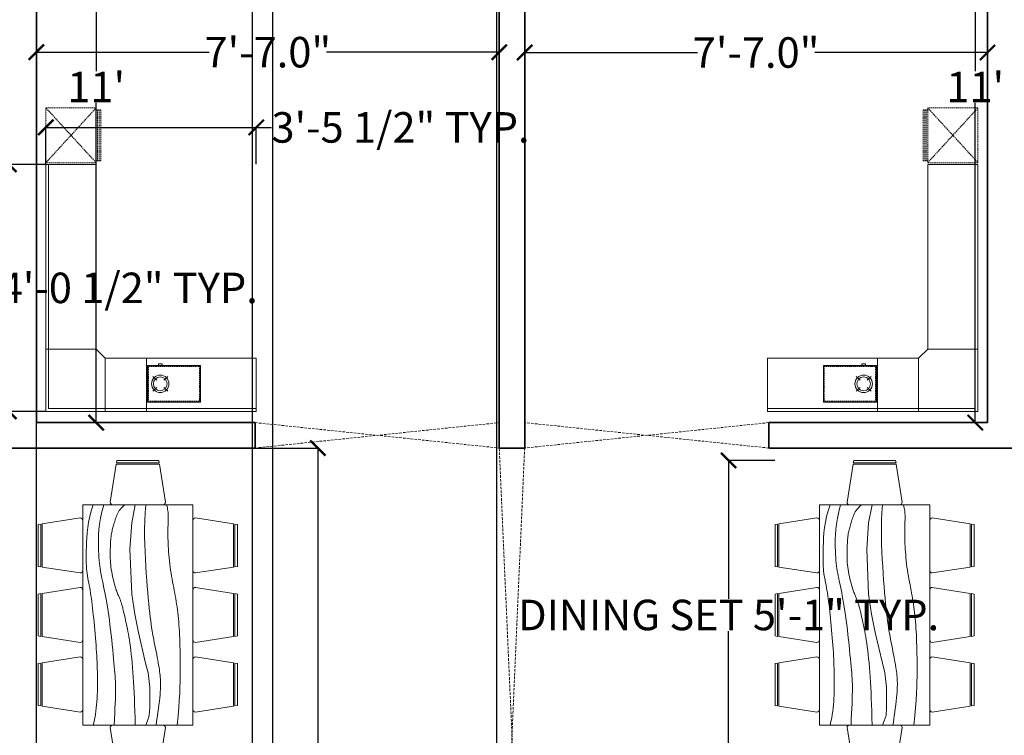
# Model space of a CAD drawing. Units: inches. Extents: x 844 to 2234, y 346 to 1084.
# Tile 44 of 93: x 1093 to 1287, y 823 to 964. Entities that reach past the tile are written whole.
import ezdxf

# ---------------------------------------------------------------- set-up
doc = ezdxf.new("R2010")
doc.units = ezdxf.units.IN
doc.header["$MEASUREMENT"] = 0
doc.linetypes.add('DASHED', pattern=[0.75, 0.5, -0.25])
doc.linetypes.add('HIDDEN', pattern=[0.375, 0.25, -0.125])
for name, color, linetype, lineweight in [('A-ANNO-DIMS', 2, 'Continuous', 18), ('A-EQPM', 42, 'Continuous', 18), ('A-EQPM-HIDN', 42, 'HIDDEN', 13), ('A-FLOR-CASE', 42, 'Continuous', 18), ('A-WALL', 7, 'Continuous', 35), ('A-WALL-OVHD', 7, 'DASHED', 18), ('furniture', 8, 'Continuous', 18)]:
    doc.layers.add(name, color=color, linetype=linetype, lineweight=lineweight)
doc.styles.add('ATTR', font='romans.shx', dxfattribs={"width": 0.8, "height": 0.7})
doc.styles.get("Standard").update_dxf_attribs({"font": 'arial.ttf'})
doc.dimstyles.get("Standard").update_dxf_attribs({"dimtxt": 6, "dimasz": 3, "dimexe": 0.18, "dimexo": 0.0625, "dimgap": 0.09, "dimtad": 0, "dimtih": 1, "dimtoh": 1, "dimdec": 1, "dimzin": 0, "dimdsep": 46, "dimlunit": 3, "dimtxsty": 'Standard', "dimblk": 'ARCHTICK', "dimcen": 0.09, "dimadec": 0, "dimazin": 0, "dimtfac": 1, "dimtdec": 1, "dimtofl": 0, "dimtmove": 0, "dimatfit": 3, "dimfxl": 1, "dimtolj": 1, "dimtzin": 0, "dimarcsym": 0})

# ---------------------------------------------------------------- blocks, each defined once
blk = doc.blocks.new('DIN42X84')
for p, q in [((-34.5377, 37.999999), (-34.6939, 37.000439)), ((-34.5377, 37.999999), (-18.5377, 37.999999)), ((-18.3814, 36.999659), (-18.5377, 37.999999)), ((-8.0001, 37.999999), (-8.1562, 37.000439)), ((-8.0001, 37.999999), (7.9999, 37.999999)), ((8.1562, 36.999659), (7.9999, 37.999999)), ((18.3813, 36.999659), (18.5376, 37.999999)), ((34.5376, 37.999999), (18.5376, 37.999999)), ((34.5376, 37.999999), (34.6938, 37.000439)), ((-34.772, 36.500609), (-37.0377, 21.999999)), ((-34.7681, 36.499999), (-18.2986, 36.499999)), ((-18.3793, 36.999999), (-34.6911, 36.999999)), ((-16.0377, 21.999999), (-18.3032, 36.499269)), ((-8.2343, 36.500609), (-10.5001, 21.999999)), ((-8.2305, 36.499999), (8.2391, 36.499999)), ((8.1584, 36.999999), (-8.1535, 36.999999)), ((10.4999, 21.999999), (8.2344, 36.499269)), ((16.0376, 21.999999), (18.3031, 36.499269)), ((34.768, 36.499999), (18.2985, 36.499999)), ((18.3792, 36.999999), (34.691, 36.999999)), ((34.7719, 36.500609), (37.0376, 21.999999)), ((-57.9997, 8.156299), (-59, 7.999989)), ((-59, -8.000011), (-59, 7.999989)), ((-58, 8.158429), (-58, -8.153391)), ((-57.5, -8.230411), (-57.5, 8.239139)), ((-43, 10.499989), (-57.4993, 8.234489)), ((43, 10.499989), (57.4992, 8.234489)), ((57.5, -8.230411), (57.5, 8.239139)), ((57.9996, 8.156299), (59, 7.999989)), ((58, 8.158429), (58, -8.153391)), ((59, -8.000011), (59, 7.999989)), ((-59, -8.000011), (-58.0005, -8.156181)), ((-57.5007, -8.234271), (-43, -10.500011)), ((57.5006, -8.234271), (43, -10.500011)), ((59, -8.000011), (58.0004, -8.156181)), ((-42, -21.000001), (42, -21.000001)), ((-34.772, -36.50061), (-37.0377, -22.000001)), ((-16.0377, -22.000001), (-18.3032, -36.499267)), ((-8.2343, -36.50061), (-10.5001, -22.000001)), ((10.4999, -22.000001), (8.2344, -36.499267)), ((16.0376, -22.000001), (18.3031, -36.499267)), ((34.7719, -36.50061), (37.0376, -22.000001)), ((-34.7681, -36.499999), (-18.2986, -36.499999)), ((-34.5377, -37.999999), (-34.6939, -37.000442)), ((-18.3793, -36.999999), (-34.6911, -36.999999)), ((-18.3814, -36.999664), (-18.5377, -37.999999)), ((-8.2305, -36.499999), (8.2391, -36.499999)), ((-8.0001, -37.999999), (-8.1562, -37.000442)), ((8.1584, -36.999999), (-8.1535, -36.999999)), ((8.1562, -36.999664), (7.9999, -37.999999)), ((34.768, -36.499999), (18.2985, -36.499999)), ((18.3792, -36.999999), (34.691, -36.999999)), ((18.3813, -36.999664), (18.5376, -37.999999)), ((34.5376, -37.999999), (34.6938, -37.000442)), ((-34.5377, -37.999999), (-18.5377, -37.999999)), ((-8.0001, -37.999999), (7.9999, -37.999999)), ((34.5376, -37.999999), (18.5376, -37.999999))]:
    blk.add_line(p, q)
for points in [[(-42, -21.000001), (-42, 20.999989), (42, 20.999989), (42, -21.000001)], [(-42, 16.999989), (-40.5974, 16.672209), (-39.2569, 16.395939), (-37.9668, 16.166109), (-36.7153, 15.977689), (-35.4906, 15.825599), (-34.281, 15.704799), (-33.0745, 15.610229), (-31.8595, 15.536839), (-30.6267, 15.480229), (-29.3778, 15.438619), (-28.117, 15.410889), (-26.8486, 15.395929), (-25.5767, 15.392599), (-24.3058, 15.399809), (-23.0399, 15.416409), (-21.7833, 15.441309), (-20.5384, 15.473619), (-19.2994, 15.513549), (-18.0587, 15.561549), (-16.8087, 15.618049), (-15.5417, 15.683499), (-14.25, 15.758369), (-12.9261, 15.843079), (-11.5622, 15.938089), (-10.1541, 16.043559), (-8.7108, 16.158419), (-7.2445, 16.281349), (-5.7675, 16.410999), (-4.2923, 16.546019), (-2.8311, 16.685069), (-1.3963, 16.826809), (0, 16.969889), (1.3474, 17.113339), (2.6447, 17.257689), (3.8928, 17.403829), (5.0924, 17.552659), (6.2444, 17.705069), (7.3498, 17.861959), (8.4092, 18.024219), (9.4237, 18.192759), (10.3952, 18.367629), (11.3311, 18.545639), (12.2397, 18.722759), (13.1297, 18.894949), (14.0095, 19.058179), (14.8876, 19.208429), (15.7725, 19.341659), (16.6727, 19.453839), (17.5977, 19.541909), (18.5617, 19.606689), (19.5795, 19.649979), (20.6664, 19.673569), (21.8374, 19.679239), (23.1076, 19.668789), (24.492, 19.644009), (26.0058, 19.606689), (27.6589, 19.554579), (29.4413, 19.469229), (31.3377, 19.328169), (33.3331, 19.108889), (35.4121, 18.788919), (37.5598, 18.345779), (39.7608, 17.756959), (42, 16.999989)], [(42, 12.999999), (39.3635, 13.704689), (36.9303, 14.232849), (34.6868, 14.608169), (32.6195, 14.854319), (30.7149, 14.994989), (28.9596, 15.053859), (27.34, 15.054629), (25.8427, 15.020959), (24.4543, 14.972439), (23.1628, 14.912279), (21.9562, 14.839589), (20.8227, 14.753449), (19.7504, 14.652989), (18.7273, 14.537299), (17.7416, 14.405489), (16.7814, 14.256669), (15.8348, 14.090369), (14.8899, 13.907959), (13.9348, 13.711209), (12.9575, 13.501929), (11.9464, 13.281899), (10.8893, 13.052909), (9.7745, 12.816759), (8.59, 12.575229), (7.3261, 12.330049), (5.9815, 12.082619), (4.557, 11.834299), (3.0536, 11.586429), (1.472, 11.340349), (-0.187, 11.097409), (-1.9223, 10.858939), (-3.7333, 10.626289), (-5.6141, 10.400739), (-7.539, 10.183249), (-9.4776, 9.974709), (-11.3991, 9.776019), (-13.2731, 9.588079), (-15.0689, 9.411789), (-16.756, 9.248039), (-18.3038, 9.097709), (-19.6928, 8.961719), (-20.9483, 8.840959), (-22.1065, 8.736319), (-23.2037, 8.648689), (-24.2763, 8.578979), (-25.3606, 8.528079), (-26.4928, 8.496879), (-27.7094, 8.486279), (-29.0411, 8.496689), (-30.4965, 8.526549), (-32.0787, 8.573829), (-33.7908, 8.636479), (-35.6359, 8.712459), (-37.6171, 8.799739), (-39.7374, 8.896259), (-42, 8.999999)], [(-42, 0.999999), (-39.2567, 1.059739), (-36.6668, 1.127399), (-34.2177, 1.203389), (-31.897, 1.288099), (-29.6923, 1.381949), (-27.5912, 1.485329), (-25.5812, 1.598659), (-23.65, 1.722319), (-21.7874, 1.856519), (-19.9935, 2.000569), (-18.2704, 2.153579), (-16.6207, 2.314649), (-15.0465, 2.482879), (-13.5503, 2.657379), (-12.1344, 2.837259), (-10.8011, 3.021619), (-9.5514, 3.209479), (-8.3812, 3.399579), (-7.2848, 3.590579), (-6.2569, 3.781129), (-5.2918, 3.969889), (-4.384, 4.155509), (-3.5281, 4.336659), (-2.7184, 4.511979), (-1.9505, 4.680359), (-1.2233, 4.841579), (-0.5369, 4.995629), (0.1087, 5.142519), (0.7135, 5.282239), (1.2776, 5.414799), (1.8009, 5.540189), (2.2834, 5.658409), (2.7259, 5.769699), (3.1323, 5.875159), (3.5073, 5.976139), (3.8555, 6.073989), (4.1816, 6.170049), (4.4904, 6.265659), (4.7863, 6.362169), (5.0742, 6.460919), (5.3584, 6.563099), (5.6417, 6.669299), (5.9267, 6.779989), (6.216, 6.895609), (6.512, 7.016589), (6.8174, 7.143399), (7.1347, 7.276479), (7.4664, 7.416279), (7.8159, 7.563169), (8.1896, 7.717219), (8.5948, 7.878439), (9.0386, 8.046819), (9.5282, 8.222369), (10.071, 8.405079), (10.674, 8.594959), (11.3446, 8.791999), (12.0866, 8.995459), (12.8902, 9.201609), (13.7421, 9.405969), (14.6294, 9.604059), (15.5387, 9.791399), (16.4569, 9.963509), (17.3709, 10.115919), (18.2674, 10.244149), (19.1361, 10.344989), (19.9772, 10.420299), (20.7936, 10.473209), (21.5884, 10.506879), (22.3645, 10.524419), (23.1248, 10.528969), (23.8725, 10.523669), (24.6103, 10.511649), (25.3403, 10.495379), (26.0601, 10.474629), (26.7663, 10.448509), (27.4556, 10.416119), (28.1244, 10.376559), (28.7695, 10.328939), (29.3873, 10.272359), (29.9746, 10.205939), (30.5293, 10.129059), (31.0552, 10.042329), (31.5572, 9.946639), (32.0406, 9.842899), (32.5104, 9.731989), (32.9716, 9.614799), (33.4295, 9.492249), (33.8891, 9.365219), (34.3546, 9.234229), (34.8266, 9.098309), (35.3051, 8.956129), (35.7897, 8.806329), (36.2802, 8.647569), (36.7765, 8.478519), (37.2783, 8.297819), (37.7854, 8.104139), (38.2976, 7.894309), (38.8146, 7.657969), (39.3361, 7.382899), (39.8617, 7.056919), (40.3912, 6.667829), (40.9243, 6.203449), (41.4607, 5.651569), (42, 4.999999)], [(42, 0.999999), (35.1214, 2.295539), (25.1178, 2.983399), (7.9376, 2.295539), (0.3261, 1.149099), (-6.6329, -0.226611), (-18.3763, -2.978061), (-22.0733, -3.895201), (-27.5101, -4.583071), (-32.9468, -4.583071), (-35.339, -4.583071), (-38.3836, -4.353771), (-40.3408, -3.665921), (-42, -3.000001)], [(42, -3.000001), (38.9344, -2.781351), (35.8829, -2.650251), (32.8567, -2.595491), (29.8672, -2.605821), (26.9257, -2.670031), (24.0436, -2.776881), (21.2323, -2.915141), (18.5031, -3.073591), (15.8668, -3.242611), (13.3327, -3.419021), (10.9095, -3.601241), (8.6059, -3.787731), (6.4305, -3.976901), (4.3921, -4.167191), (2.4994, -4.357031), (0.7611, -4.544851), (-0.8196, -4.729651), (-2.2614, -4.912671), (-3.5885, -5.095681), (-4.8252, -5.280481), (-5.9956, -5.468861), (-7.1239, -5.662621), (-8.2344, -5.863551), (-9.3513, -6.073431), (-10.4925, -6.293091), (-11.6511, -6.519461), (-12.814, -6.748531), (-13.968, -6.976251), (-15.0999, -7.198591), (-16.1965, -7.411531), (-17.2447, -7.611041), (-18.2313, -7.793081), (-19.1472, -7.954521), (-19.9994, -8.095811), (-20.7989, -8.218291), (-21.5568, -8.323311), (-22.2841, -8.412201), (-22.9919, -8.486311), (-23.6912, -8.546991), (-24.393, -8.595581), (-25.1087, -8.632751), (-25.8513, -8.656491), (-26.6337, -8.664101), (-27.4693, -8.652901), (-28.3711, -8.620211), (-29.3523, -8.563341), (-30.4262, -8.479601), (-31.6057, -8.366301), (-32.8956, -8.222561), (-34.2657, -8.054761), (-35.6772, -7.871051), (-37.0913, -7.679611), (-38.4695, -7.488621), (-39.7728, -7.306241), (-40.9626, -7.140641), (-42, -7.000001)], [(-42, -15.000001), (-38.4722, -15.350691), (-35.3039, -15.623741), (-32.4544, -15.828971), (-29.8831, -15.976191), (-27.5493, -16.075201), (-25.4123, -16.135831), (-23.4313, -16.167881), (-21.5659, -16.181151), (-19.7812, -16.183881), (-18.0665, -16.177871), (-16.4173, -16.163351), (-14.8288, -16.140551), (-13.2964, -16.109691), (-11.8154, -16.070991), (-10.3811, -16.024671), (-8.9888, -15.970971), (-7.6345, -15.909991), (-6.3163, -15.841401), (-5.0329, -15.764751), (-3.7831, -15.679591), (-2.5656, -15.585471), (-1.3791, -15.481951), (-0.2223, -15.368571), (0.9061, -15.244901), (2.0079, -15.110631), (3.0876, -14.966051), (4.1503, -14.811631), (5.2011, -14.647801), (6.2451, -14.475011), (7.2875, -14.293721), (8.3332, -14.104361), (9.3874, -13.907391), (10.4544, -13.703711), (11.5349, -13.495991), (12.6291, -13.287381), (13.7368, -13.081011), (14.8581, -12.880011), (15.9931, -12.687521), (17.1416, -12.506671), (18.3037, -12.340601), (19.4778, -12.191771), (20.6562, -12.059961), (21.8295, -11.944271), (22.9884, -11.843811), (24.1234, -11.757681), (25.2254, -11.684981), (26.2848, -11.624831), (27.2925, -11.576311), (28.2412, -11.538551), (29.1325, -11.510631), (29.9703, -11.491671), (30.7584, -11.480781), (31.5007, -11.477041), (32.2009, -11.479581), (32.8628, -11.487491), (33.4904, -11.499881), (34.0874, -11.515741), (34.6576, -11.533621), (35.2049, -11.551941), (35.733, -11.569151), (36.2459, -11.583661), (36.7473, -11.593931), (37.2411, -11.598371), (37.7311, -11.595421), (38.2211, -11.583281), (38.7152, -11.559251), (39.2177, -11.520361), (39.7326, -11.463671), (40.2641, -11.386241), (40.8164, -11.285111), (41.3937, -11.157351), (42, -11.000001)]]:
    blk.add_lwpolyline(points)
for centre, start, end in [((-36.0377, 21.999999), 180, 270), ((-17.0377, 21.999999), 270, 0), ((-9.5001, 21.999999), 180, 270), ((9.4999, 21.999999), 270, 0), ((17.0376, 21.999999), 180, 270), ((36.0376, 21.999999), 270, 0), ((-43, 9.499989), 0.00000068, 90), ((43, 9.499989), 90, 180), ((-43, -9.500011), 270, 0.00000068), ((43, -9.500011), 180, 270), ((-36.0377, -22.000001), 90, 180), ((-17.0377, -22.000001), 0, 90), ((-9.5001, -22.000001), 90, 180), ((9.4999, -22.000001), 0, 90), ((17.0376, -22.000001), 90, 180), ((36.0376, -22.000001), 0, 90)]:
    blk.add_arc(centre, 1, start, end)
at = {"style": 'ATTR', "width": 0.8, "flags": 9}
blk.add_attdef('ESTCODE', (0, 0), '', height=0.7, dxfattribs=at)
blk = doc.blocks.new('_ArchTick')
at = {"color": 0, "linetype": 'ByBlock', "const_width": 0.15}
blk.add_lwpolyline([(-0.5, -0.5), (0.5, 0.5)], dxfattribs=at)
blk = doc.blocks.new('*D25')
at = {"layer": 'A-ANNO-DIMS', "color": 0, "lineweight": -2, "transparency": 16777216}
for p, q in [((1096.62, 957.17), (1130.58, 957.17)), ((1096.62, 957.1), (1096.62, 956.99)), ((1187.62, 957.17), (1153.65, 957.17)), ((1187.62, 957.23), (1187.62, 957.35))]:
    blk.add_line(p, q, dxfattribs=at)
at = {"layer": 'Defpoints', "color": 0, "transparency": 16777216}
for p in [(1096.62, 957.17), (1187.62, 957.17), (1187.62, 957.17)]:
    blk.add_point(p, dxfattribs=at)
at = {"layer": 'A-ANNO-DIMS', "color": 0, "lineweight": -2, "transparency": 16777216, "xscale": 3, "yscale": 3, "zscale": 3, "rotation": 180}
blk.add_blockref('_ArchTick', (1096.62, 957.17), dxfattribs=at)
at = {"layer": 'A-ANNO-DIMS', "color": 0, "lineweight": -2, "transparency": 16777216, "xscale": 3, "yscale": 3, "zscale": 3}
blk.add_blockref('_ArchTick', (1187.62, 957.17), dxfattribs=at)
at = {"layer": 'A-ANNO-DIMS', "color": 0, "transparency": 16777216, "insert": (1142.12, 957.17), "char_height": 6, "attachment_point": 5}
blk.add_mtext('\\A1;7\'-7.0"', dxfattribs=at)
blk = doc.blocks.new('*D26')
at = {"layer": 'A-ANNO-DIMS', "color": 0, "lineweight": -2, "transparency": 16777216}
for p, q in [((1099.7, 1016.31), (1108.56, 1016.31)), ((1108.38, 1016.31), (1108.38, 953.41)), ((1108.38, 884.31), (1108.38, 947.21)), ((1099.7, 884.31), (1108.56, 884.31))]:
    blk.add_line(p, q, dxfattribs=at)
at = {"layer": 'Defpoints', "color": 0, "transparency": 16777216}
for p in [(1099.64, 1016.31), (1099.64, 884.31), (1108.38, 884.31)]:
    blk.add_point(p, dxfattribs=at)
at = {"layer": 'A-ANNO-DIMS', "color": 0, "lineweight": -2, "transparency": 16777216, "xscale": 3, "yscale": 3, "zscale": 3}
for p, rotation in [((1108.38, 1016.31), 90), ((1108.38, 884.31), 270)]:
    blk.add_blockref('_ArchTick', p, dxfattribs=dict(at, rotation=rotation))
at = {"layer": 'A-ANNO-DIMS', "color": 0, "transparency": 16777216, "insert": (1108.38, 950.31), "char_height": 6, "attachment_point": 5}
blk.add_mtext("\\A1;11'", dxfattribs=at)
blk = doc.blocks.new('*D27')
at = {"layer": 'A-ANNO-DIMS', "color": 0, "lineweight": -2, "transparency": 16777216}
for p, q in [((1283.21, 1016.31), (1281.03, 1016.31)), ((1281.21, 1016.31), (1281.21, 953.41)), ((1281.21, 884.31), (1281.21, 947.21)), ((1283.21, 884.31), (1281.03, 884.31))]:
    blk.add_line(p, q, dxfattribs=at)
at = {"layer": 'Defpoints', "color": 0, "transparency": 16777216}
for p in [(1283.27, 1016.31), (1281.21, 884.31), (1283.27, 884.31)]:
    blk.add_point(p, dxfattribs=at)
at = {"layer": 'A-ANNO-DIMS', "color": 0, "lineweight": -2, "transparency": 16777216, "xscale": 3, "yscale": 3, "zscale": 3}
for p, rotation in [((1281.21, 1016.31), 90), ((1281.21, 884.31), 270)]:
    blk.add_blockref('_ArchTick', p, dxfattribs=dict(at, rotation=rotation))
at = {"layer": 'A-ANNO-DIMS', "color": 0, "transparency": 16777216, "insert": (1281.21, 950.31), "char_height": 6, "attachment_point": 5}
blk.add_mtext("\\A1;11'", dxfattribs=at)
blk = doc.blocks.new('*D28')
at = {"layer": 'A-ANNO-DIMS', "color": 0, "lineweight": -2, "transparency": 16777216}
for p, q in [((1192.62, 957.17), (1192.62, 957.28)), ((1192.62, 957.1), (1226.58, 957.1)), ((1283.62, 957.1), (1249.65, 957.1)), ((1283.62, 957.17), (1283.62, 957.28))]:
    blk.add_line(p, q, dxfattribs=at)
at = {"layer": 'Defpoints', "color": 0, "transparency": 16777216}
for p in [(1192.62, 957.1), (1283.62, 957.1), (1283.62, 957.1)]:
    blk.add_point(p, dxfattribs=at)
at = {"layer": 'A-ANNO-DIMS', "color": 0, "lineweight": -2, "transparency": 16777216, "xscale": 3, "yscale": 3, "zscale": 3, "rotation": 180}
blk.add_blockref('_ArchTick', (1192.62, 957.1), dxfattribs=at)
at = {"layer": 'A-ANNO-DIMS', "color": 0, "lineweight": -2, "transparency": 16777216, "xscale": 3, "yscale": 3, "zscale": 3}
blk.add_blockref('_ArchTick', (1283.62, 957.1), dxfattribs=at)
at = {"layer": 'A-ANNO-DIMS', "color": 0, "transparency": 16777216, "insert": (1238.12, 957.1), "char_height": 6, "attachment_point": 5}
blk.add_mtext('\\A1;7\'-7.0"', dxfattribs=at)
blk = doc.blocks.new('*D54')
at = {"layer": 'A-ANNO-DIMS', "color": 0, "lineweight": -2, "transparency": 16777216}
for p, q in [((1139.68, 879.31), (1152.12, 879.31)), ((1151.94, 879.31), (1151.94, 758.4)), ((1151.94, 631.18), (1151.94, 752.09)), ((1139.68, 631.18), (1152.12, 631.18))]:
    blk.add_line(p, q, dxfattribs=at)
at = {"layer": 'Defpoints', "color": 0, "transparency": 16777216}
for p in [(1139.62, 879.31), (1139.62, 631.18), (1151.94, 631.18)]:
    blk.add_point(p, dxfattribs=at)
at = {"layer": 'A-ANNO-DIMS', "color": 0, "lineweight": -2, "transparency": 16777216, "xscale": 3, "yscale": 3, "zscale": 3}
for p, rotation in [((1151.94, 879.31), 90), ((1151.94, 631.18), 270)]:
    blk.add_blockref('_ArchTick', p, dxfattribs=dict(at, rotation=rotation))
at = {"layer": 'A-ANNO-DIMS', "color": 0, "transparency": 16777216, "insert": (1151.94, 755.25), "char_height": 6, "attachment_point": 5}
blk.add_mtext('\\A1;20\'-8.1"', dxfattribs=at)
blk = doc.blocks.new('KITCHEN-TALL-UNIT-COMPACT')
for p, q in [((9.89, 0), (0, 10.79)), ((9.89, 10.79), (0, 0)), ((10.18, 0.36), (10.18, 10.43)), ((10.48, 0.36), (10.48, 10.43))]:
    blk.add_line(p, q)
blk.add_lwpolyline([(9.89, 0), (0, 0), (0, 10.79), (9.89, 10.79)], close=True)
blk.add_lwpolyline([(9.89, 0.36), (10.79, 0.36), (10.79, 10.43), (9.89, 10.43)])
blk = doc.blocks.new('KITCHEN-COUNTER-L')
for p, q in [((0, 0), (0, 48.56)), ((0, 48.56), (9.89, 48.56)), ((0.54, 0.54), (0.54, 48.56)), ((9.89, 12.23), (9.89, 48.56)), ((9.89, 12.23), (0, 12.23)), ((11.69, 10.43), (9.89, 12.23)), ((11.69, 10.43), (11.69, 0)), ((11.69, 10.43), (41.36, 10.43)), ((19.78, 0), (19.78, 10.43)), ((41.36, 0), (41.36, 10.43)), ((0.54, 0.54), (41.36, 0.54)), ((0, 0), (41.36, 0)), ((0, 0), (9.89, 0))]:
    blk.add_line(p, q)
blk = doc.blocks.new('HOB-1-BURNER')
for p, q in [((1.82, 4.31), (1.06, 5.08)), ((3.98, 5.08), (3.22, 4.31)), ((1.82, 2.92), (1.06, 2.15)), ((3.98, 2.15), (3.22, 2.92))]:
    blk.add_line(p, q)
blk.add_lwpolyline([(10.43, 0), (10.43, 7.19), (0, 7.19), (0, 0)], close=True)
blk.add_lwpolyline([(2.88, 7.19), (2.88, 7.55), (2.16, 7.55), (2.16, 7.18)])
for radius in [1.71, 1.35]:
    blk.add_circle((2.52, 3.61), radius)
blk = doc.blocks.new('*D119')
at = {"layer": 'A-ANNO-DIMS', "color": 0, "lineweight": -2, "transparency": 16777216}
for p, q in [((1241.78, 876.89), (1232.54, 876.89)), ((1232.72, 876.89), (1232.72, 849.68)), ((1232.72, 816.08), (1232.72, 843.29)), ((1241.78, 816.08), (1232.54, 816.08))]:
    blk.add_line(p, q, dxfattribs=at)
at = {"layer": 'Defpoints', "color": 0, "transparency": 16777216}
for p in [(1232.72, 876.89), (1241.84, 876.89), (1241.84, 816.08)]:
    blk.add_point(p, dxfattribs=at)
at = {"layer": 'A-ANNO-DIMS', "color": 0, "lineweight": -2, "transparency": 16777216, "xscale": 3, "yscale": 3, "zscale": 3}
for p, rotation in [((1232.72, 876.89), 90), ((1232.72, 816.08), 270)]:
    blk.add_blockref('_ArchTick', p, dxfattribs=dict(at, rotation=rotation))
at = {"layer": 'A-ANNO-DIMS', "color": 0, "transparency": 16777216, "insert": (1232.72, 846.48), "char_height": 6, "attachment_point": 5}
blk.add_mtext('\\A1;DINING SET 5\'-1" TYP.', dxfattribs=at)
blk = doc.blocks.new('*D131')
at = {"layer": 'A-ANNO-DIMS', "color": 0, "lineweight": -2, "transparency": 16777216}
for p, q in [((1098.42, 935.09), (1091.02, 935.09)), ((1091.2, 935.09), (1091.2, 914)), ((1091.2, 886.53), (1091.2, 907.62)), ((1098.42, 886.53), (1091.02, 886.53))]:
    blk.add_line(p, q, dxfattribs=at)
at = {"layer": 'Defpoints', "color": 0, "transparency": 16777216}
for p in [(1091.2, 935.09), (1098.48, 935.09), (1098.48, 886.53)]:
    blk.add_point(p, dxfattribs=at)
at = {"layer": 'A-ANNO-DIMS', "color": 0, "lineweight": -2, "transparency": 16777216, "xscale": 3, "yscale": 3, "zscale": 3}
for p, rotation in [((1091.2, 935.09), 90), ((1091.2, 886.53), 270)]:
    blk.add_blockref('_ArchTick', p, dxfattribs=dict(at, rotation=rotation))
at = {"layer": 'A-ANNO-DIMS', "color": 0, "transparency": 16777216, "insert": (1091.2, 910.81), "char_height": 6, "attachment_point": 5}
blk.add_mtext('\\A1;L-COUNTER 4\'-0 1/2" TYP.', dxfattribs=at)
blk = doc.blocks.new('*D132')
at = {"layer": 'A-ANNO-DIMS', "color": 0, "lineweight": -2, "transparency": 16777216}
for p, q in [((1098.48, 935.15), (1098.48, 942.55)), ((1098.48, 942.37), (1139.85, 942.37)), ((1139.85, 935.15), (1139.85, 942.55)), ((1139.85, 942.37), (1142.85, 942.37))]:
    blk.add_line(p, q, dxfattribs=at)
at = {"layer": 'Defpoints', "color": 0, "transparency": 16777216}
for p in [(1139.85, 942.37), (1098.48, 935.09), (1139.85, 935.09)]:
    blk.add_point(p, dxfattribs=at)
at = {"layer": 'A-ANNO-DIMS', "color": 0, "lineweight": -2, "transparency": 16777216, "xscale": 3, "yscale": 3, "zscale": 3, "rotation": 180}
blk.add_blockref('_ArchTick', (1098.48, 942.37), dxfattribs=at)
at = {"layer": 'A-ANNO-DIMS', "color": 0, "lineweight": -2, "transparency": 16777216, "xscale": 3, "yscale": 3, "zscale": 3}
blk.add_blockref('_ArchTick', (1139.85, 942.37), dxfattribs=at)
at = {"layer": 'A-ANNO-DIMS', "color": 0, "transparency": 16777216, "insert": (1168.21, 942.37), "char_height": 6, "attachment_point": 5}
blk.add_mtext('\\A1;3\'-5 1/2" TYP.', dxfattribs=at)
blk = doc.blocks.new('*D143')
at = {"layer": 'A-ANNO-DIMS', "color": 0, "lineweight": -2, "transparency": 16777216}
for p, q in [((1139.12, 430.37), (1139.12, 1074.74)), ((1139.12, 1074.56), (1154.93, 1074.56)), ((1187.12, 1074.56), (1171.3, 1074.56)), ((1187.12, 430.37), (1187.12, 1074.74))]:
    blk.add_line(p, q, dxfattribs=at)
at = {"layer": 'Defpoints', "color": 0, "transparency": 16777216}
for p in [(1187.12, 1074.56), (1139.12, 430.31), (1187.12, 430.31)]:
    blk.add_point(p, dxfattribs=at)
at = {"layer": 'A-ANNO-DIMS', "color": 0, "lineweight": -2, "transparency": 16777216, "xscale": 3, "yscale": 3, "zscale": 3, "rotation": 180}
blk.add_blockref('_ArchTick', (1139.12, 1074.56), dxfattribs=at)
at = {"layer": 'A-ANNO-DIMS', "color": 0, "lineweight": -2, "transparency": 16777216, "xscale": 3, "yscale": 3, "zscale": 3}
blk.add_blockref('_ArchTick', (1187.12, 1074.56), dxfattribs=at)
at = {"layer": 'A-ANNO-DIMS', "color": 0, "transparency": 16777216, "insert": (1163.12, 1074.56), "char_height": 6, "attachment_point": 5}
blk.add_mtext('\\A1;4\'-0"', dxfattribs=at)
blk = doc.blocks.new('*D144')
at = {"layer": 'A-ANNO-DIMS', "color": 0, "lineweight": -2, "transparency": 16777216}
for p, q in [((1096.62, 439.37), (1096.62, 1074.74)), ((1096.62, 1074.56), (1102.48, 1074.56)), ((1143.12, 1074.56), (1137.25, 1074.56)), ((1143.12, 492.37), (1143.12, 1074.74))]:
    blk.add_line(p, q, dxfattribs=at)
at = {"layer": 'Defpoints', "color": 0, "transparency": 16777216}
for p in [(1143.12, 1074.56), (1143.12, 492.31), (1096.62, 439.31)]:
    blk.add_point(p, dxfattribs=at)
at = {"layer": 'A-ANNO-DIMS', "color": 0, "lineweight": -2, "transparency": 16777216, "xscale": 3, "yscale": 3, "zscale": 3, "rotation": 180}
blk.add_blockref('_ArchTick', (1096.62, 1074.56), dxfattribs=at)
at = {"layer": 'A-ANNO-DIMS', "color": 0, "lineweight": -2, "transparency": 16777216, "xscale": 3, "yscale": 3, "zscale": 3}
blk.add_blockref('_ArchTick', (1143.12, 1074.56), dxfattribs=at)
at = {"layer": 'A-ANNO-DIMS', "color": 0, "transparency": 16777216, "insert": (1119.87, 1074.56), "char_height": 6, "attachment_point": 5}
blk.add_mtext('\\A1;3\'-10 1/2"', dxfattribs=at)

msp = doc.modelspace()

# ---------------------------------------------------------------- linework, layer by layer
at = {"layer": 'A-EQPM-HIDN'}
for points in [[(1128.7, 888.51), (1128.7, 895.34), (1118.63, 895.34), (1118.63, 888.51)], [(1251.53, 888.51), (1251.53, 895.34), (1261.61, 895.34), (1261.61, 888.51)]]:
    msp.add_lwpolyline(points, close=True, dxfattribs=at)
at = {"layer": 'A-WALL'}
for p, q in [((1096.62, 1016.31), (1096.62, 884.31)), ((1187.62, 1016.31), (1187.62, 884.31)), ((1192.62, 1016.31), (1192.62, 884.31)), ((1283.62, 1016.31), (1283.62, 884.31)), ((1096.62, 884.31), (1139.62, 884.31)), ((1139.62, 884.31), (1139.62, 879.31)), ((1187.62, 884.31), (1187.62, 879.31)), ((1192.62, 884.31), (1192.62, 879.31)), ((1240.62, 884.31), (1283.62, 884.31)), ((1240.62, 884.31), (1240.62, 879.31)), ((1087.62, 879.31), (1139.62, 879.31)), ((1187.62, 879.31), (1192.62, 879.31)), ((1240.62, 879.31), (1292.62, 879.31))]:
    msp.add_line(p, q, dxfattribs=at)
at = {"layer": 'A-WALL-OVHD'}
for p, q in [((1139.62, 884.31), (1187.62, 879.31)), ((1139.62, 879.31), (1187.62, 884.31)), ((1240.62, 884.31), (1192.62, 879.31)), ((1240.62, 879.31), (1192.62, 884.31)), ((1192.62, 766.31), (1187.62, 879.31)), ((1192.62, 879.31), (1187.62, 766.31))]:
    msp.add_line(p, q, dxfattribs=at)

# ---------------------------------------------------------------- block references
at = {"layer": 'A-EQPM'}
msp.add_blockref('HOB-1-BURNER', (1118.45, 888.33), dxfattribs=at)
at = {"layer": 'A-EQPM', "extrusion": (0, 0, -1), "zscale": -1}
msp.add_blockref('HOB-1-BURNER', (-1261.79, 888.33), dxfattribs=at)
at = {"layer": 'A-EQPM-HIDN'}
msp.add_blockref('KITCHEN-TALL-UNIT-COMPACT', (1098.48, 935.43), dxfattribs=at)
at = {"layer": 'A-EQPM-HIDN', "extrusion": (0, 0, -1), "zscale": -1}
msp.add_blockref('KITCHEN-TALL-UNIT-COMPACT', (-1281.75, 935.43), dxfattribs=at)
at = {"layer": 'A-FLOR-CASE'}
msp.add_blockref('KITCHEN-COUNTER-L', (1098.48, 886.53), dxfattribs=at)
at = {"layer": 'A-FLOR-CASE', "extrusion": (0, 0, -1), "zscale": -1}
msp.add_blockref('KITCHEN-COUNTER-L', (-1281.75, 886.53), dxfattribs=at)
at = {"layer": 'furniture', "xscale": 0.5153672157522483, "yscale": 0.5153672157522483, "zscale": 0.5153672157522483, "rotation": 90}
for p in [(1116.56, 846.48), (1261.43, 846.48)]:
    msp.add_blockref('DIN42X84', p, dxfattribs=at)

# ---------------------------------------------------------------- dimensions: what is measured, and where the dimension line sits
at = {"layer": 'A-ANNO-DIMS'}
for base, p1, p2, override, picture, middle in [((1143.12, 1074.56), (1096.62, 439.31), (1143.12, 492.31), {"dimdec": 1, "dimlfac": 1, "dimrnd": 0, "dimzin": 1, "dimdsep": 46, "dimlunit": 4, "dimfrac": 2}, '*D144', (1119.87, 1074.56)), ((1187.12, 1074.56), (1139.12, 430.31), (1187.12, 430.31), {"dimdec": 1, "dimlfac": 1, "dimrnd": 0, "dimzin": 1, "dimdsep": 46, "dimlunit": 4, "dimfrac": 2}, '*D143', (1163.12, 1074.56)), ((1187.62, 957.17), (1096.62, 957.17), (1187.62, 957.17), {"dimclrd": 0, "dimclre": 0, "dimclrt": 0}, '*D25', (1142.12, 957.17)), ((1283.62, 957.1), (1192.62, 957.1), (1283.62, 957.1), {"dimclrd": 0, "dimclre": 0, "dimclrt": 0}, '*D28', (1238.12, 957.1))]:
    dim = msp.add_linear_dim(base=base, p1=p1, p2=p2, dimstyle='Standard', override=override, dxfattribs=at)
    dim.commit()
    dim.dimension.update_dxf_attribs({"geometry": picture, "text_midpoint": middle})
for base, p1, p2, picture, middle in [((1108.38, 884.31), (1099.64, 1016.31), (1099.64, 884.31), '*D26', (1108.38, 950.31)), ((1281.21, 884.31), (1283.27, 1016.31), (1283.27, 884.31), '*D27', (1281.21, 950.31)), ((1151.94, 631.18), (1139.62, 879.31), (1139.62, 631.18), '*D54', (1151.94, 755.25))]:
    dim = msp.add_linear_dim(base=base, p1=p1, p2=p2, angle=90, dimstyle='Standard', override={"dimclrd": 0, "dimclre": 0, "dimclrt": 0}, dxfattribs=at)
    dim.commit()
    dim.dimension.update_dxf_attribs({"geometry": picture, "text_midpoint": middle})
dim = msp.add_linear_dim(base=(1139.85, 942.37), p1=(1098.48, 935.09), p2=(1139.85, 935.09), text='<> TYP.', dimstyle='Standard', override={"dimdec": 1, "dimlfac": 1, "dimrnd": 0, "dimzin": 1, "dimdsep": 46, "dimlunit": 4, "dimfrac": 2}, dxfattribs=at)
dim.commit()
dim.dimension.update_dxf_attribs({"geometry": '*D132', "text_midpoint": (1168.21, 942.37)})
for base, p1, p2, text, picture, middle in [((1091.2, 935.09), (1098.48, 886.53), (1098.48, 935.09), 'L-COUNTER <> TYP.', '*D131', (1091.2, 910.81)), ((1232.72, 876.89), (1241.84, 816.08), (1241.84, 876.89), 'DINING SET <> TYP.', '*D119', (1232.72, 846.48))]:
    dim = msp.add_linear_dim(base=base, p1=p1, p2=p2, angle=90, text=text, dimstyle='Standard', override={"dimdec": 1, "dimlfac": 1, "dimrnd": 0, "dimzin": 1, "dimdsep": 46, "dimlunit": 4, "dimfrac": 2}, dxfattribs=at)
    dim.commit()
    dim.dimension.update_dxf_attribs({"geometry": picture, "text_midpoint": middle})

doc.saveas('drawing.dxf')
